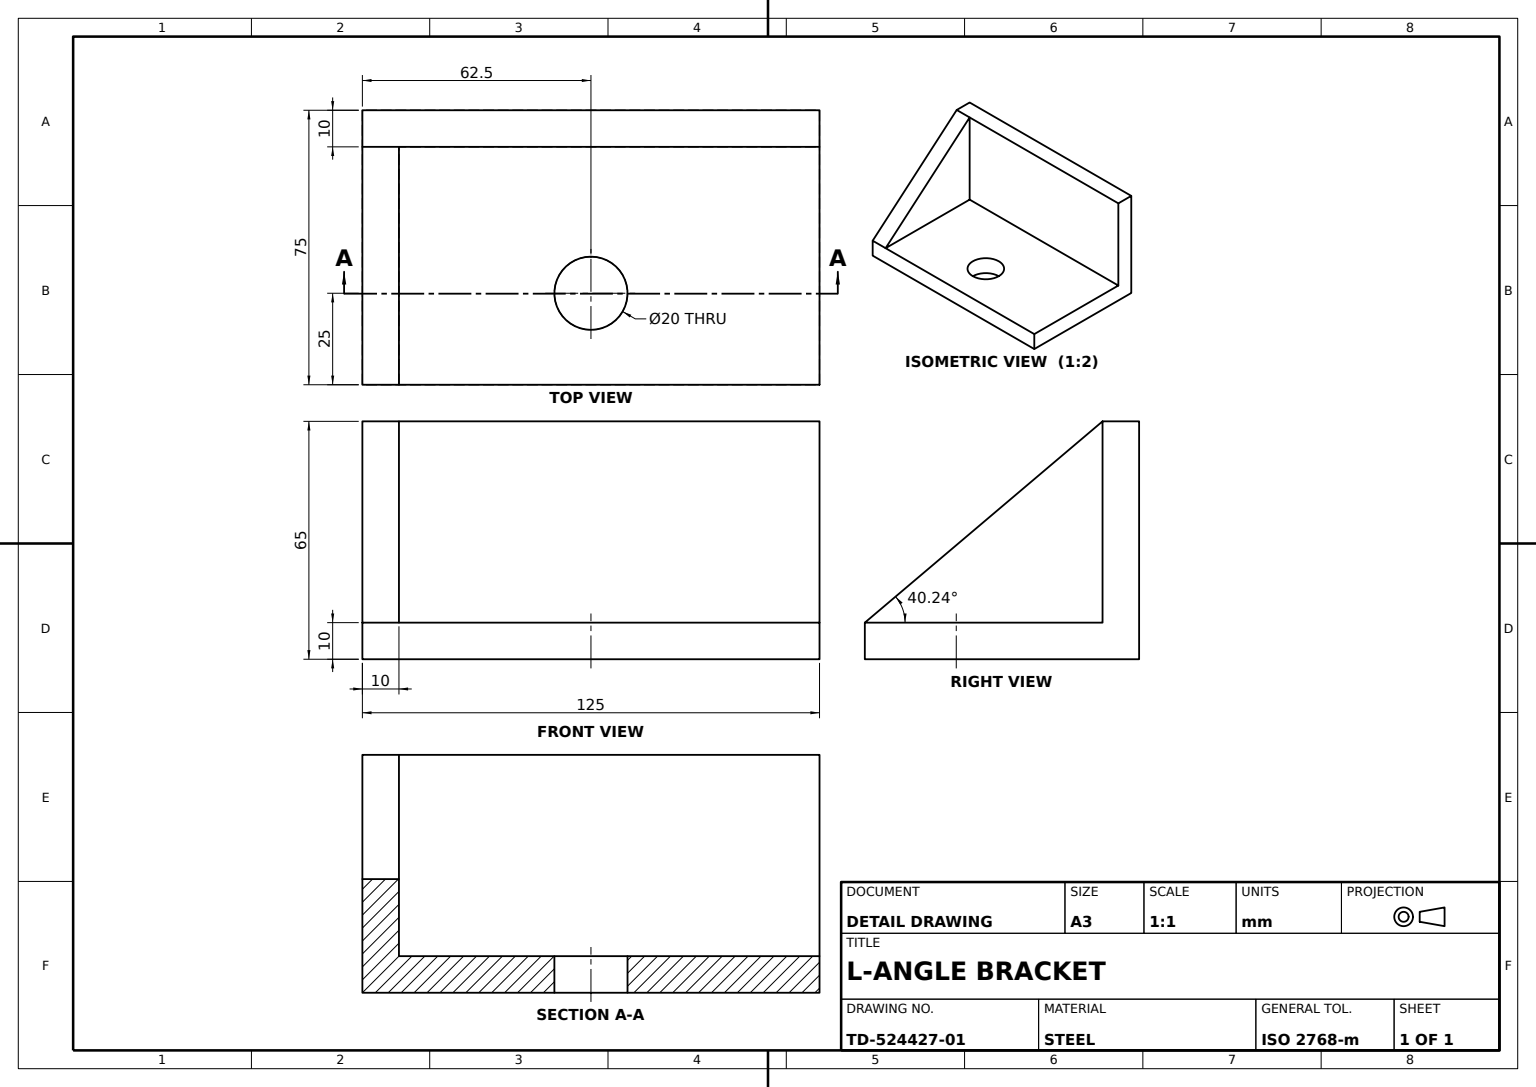
from build123d import *

# Parameters (mm, degrees)
BASE_PLATE_PROFILE_W  = 125
BASE_PLATE_PROFILE_H  = 10
BASE_PLATE_DEPTH      = 75
BACK_WALL_PROFILE_W   = 125
BACK_WALL_PROFILE_H   = 10
BACK_WALL_DEPTH       = 55
END_WALL_PROFILE_W    = 10
END_WALL_PROFILE_H    = 65
END_WALL_DEPTH        = 55
GUSSET_TRIM_CUT_DEPTH = 55
BASE_HOLE_20_SKETCH_R = 10
BASE_HOLE_20_DEPTH    = 55


with BuildPart() as part:
    # Base Plate Profile → Base Plate (new body)
    with BuildSketch(Plane.XY):
        with Locations((62.5, 5)):
            Rectangle(BASE_PLATE_PROFILE_W, BASE_PLATE_PROFILE_H)
    extrude(amount=BASE_PLATE_DEPTH)

    # Back Wall Profile → Back Wall (add)
    with BuildSketch(Plane(origin=(0, 10, 0), x_dir=(1, 0, 0), z_dir=(0, 1, 0))):
        with Locations((62.5, -5)):
            Rectangle(BACK_WALL_PROFILE_W, BACK_WALL_PROFILE_H)
    extrude(amount=BACK_WALL_DEPTH)

    # End Wall Profile → End Wall (add)
    with BuildSketch(Plane(origin=(0, 10, 0), x_dir=(1, 0, 0), z_dir=(0, 1, 0))):
        with Locations((5, -42.5)):
            Rectangle(END_WALL_PROFILE_W, END_WALL_PROFILE_H)
    extrude(amount=END_WALL_DEPTH)

    # Gusset Trim Profile → Gusset Trim Cut (cut)
    with BuildSketch(Plane(origin=(10, 0, 0), x_dir=(0, 0, -1), z_dir=(1, 0, 0))):
        Polygon((-10, 65), (-75, 10), (-75, 65), align=None)
    extrude(amount=-GUSSET_TRIM_CUT_DEPTH, mode=Mode.SUBTRACT)

    # Base Hole Ø20 Sketch → Base Hole Ø20 (cut)
    with BuildSketch(Plane(origin=(0, 10, 0), x_dir=(1, 0, 0), z_dir=(0, 1, 0))):
        with Locations(Location((62.5, -50, 0), (0, 0, 270))):
            Circle(BASE_HOLE_20_SKETCH_R)
    extrude(amount=-BASE_HOLE_20_DEPTH, mode=Mode.SUBTRACT)


solid = part.part
